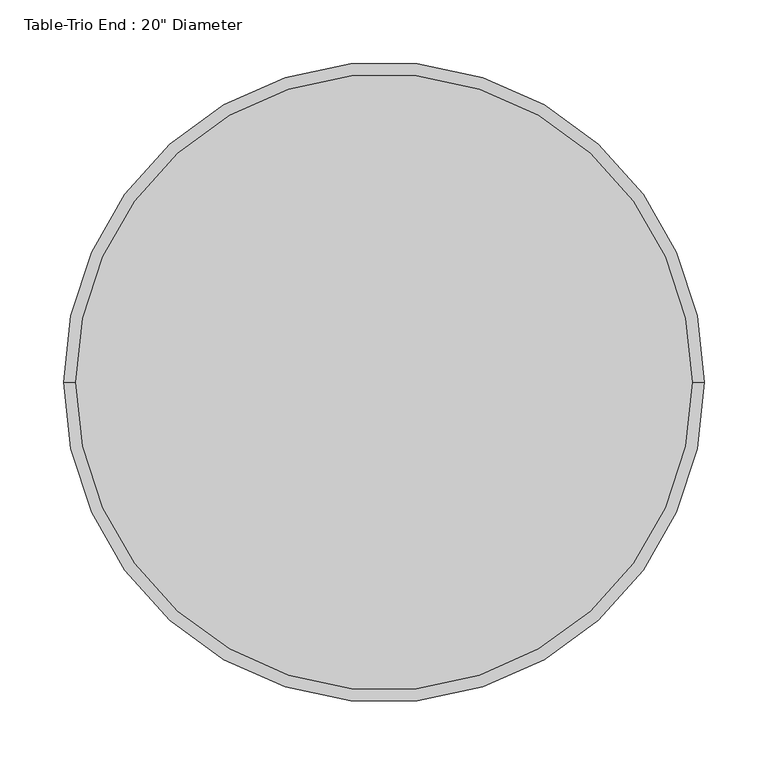
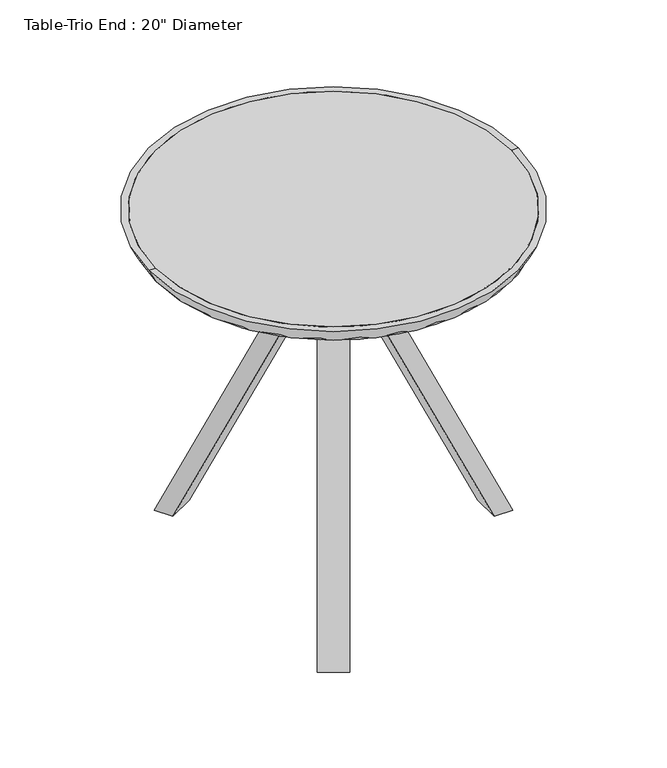
"""IFC4 building model written with IfcOpenShell, lengths in millimetres: furniture geometry."""

from ifc_helpers import new_model, si_unit, point, frame, frame_2d, origin, origin_2d, place, context, project, spatial, polyline, circle_curve, trimmed, segment, composite_curve, outline, extrude, source, transform, mapped, element, save
from ifc_brep_helpers import plane_surface, revolved_surface, advanced_brep


def furniture_3dd5e188(model_context):
    return source(origin(), model_context, "Body", "SolidModel", [
        extrude(outline(composite_curve([segment(trimmed(circle_curve(origin_2d(), 241.3), [point((-241.3, 0.0))], [point((241.3, 0.0))], False, "CARTESIAN"), True, "CONTINUOUS"), segment(trimmed(circle_curve(origin_2d(), 241.3), [point((241.3, 0.0))], [point((-241.3, 0.0))], False, "CARTESIAN"), True, "CONTINUOUS")], self_intersect=False)), frame((0.0, 0.0, 482.6), z_axis=(0.0, 0.0, 1.0), x_axis=(1.0, 0.0, 0.0)), (0.0, 0.0, 1.0), 19.05),
        advanced_brep(
        [(241.3, 0.0, 482.6), (241.3, 0.0, 501.65), (-241.3, 0.0, 501.65), (-241.3, 0.0, 482.6), (250.825, 0.0, 501.65), (-250.825, 0.0, 501.65)],
        [
            (0, 1),
            (1, 2, circle_curve(frame((0.0, 0.0, 501.65), z_axis=(0.0, 0.0, 1.0), x_axis=(-1.0, 0.0, 0.0)), 241.3)),
            (2, 3),
            (3, 0, circle_curve(frame((0.0, 0.0, 482.6), z_axis=(0.0, 0.0, -1.0), x_axis=(-1.0, 0.0, 0.0)), 241.3)),
            (4, 0),
            (3, 5),
            (5, 4, circle_curve(frame((0.0, 0.0, 501.65), z_axis=(0.0, 0.0, -1.0), x_axis=(-1.0, 0.0, 0.0)), 250.825)),
            (1, 4),
            (5, 2),
            (2, 1, circle_curve(frame((0.0, 0.0, 501.65), z_axis=(0.0, 0.0, 1.0), x_axis=(1.0, 0.0, 0.0)), 241.3)),
            (0, 3, circle_curve(frame((0.0, 0.0, 482.6), z_axis=(0.0, 0.0, -1.0), x_axis=(1.0, 0.0, 0.0)), 241.3)),
            (4, 5, circle_curve(frame((0.0, 0.0, 501.65), z_axis=(0.0, 0.0, -1.0), x_axis=(1.0, 0.0, 0.0)), 250.825)),
        ],
        [
            revolved_surface(polyline([(-241.3, 0.0, 501.65), (-241.3, 0.0, 482.6)]), (0.0, 0.0, 0.0), (0.0, 0.0, 1.0)),
            revolved_surface(polyline([(-241.3, 0.0, 482.6), (-250.825, 0.0, 501.65)]), (0.0, 0.0, 0.0), (0.0, 0.0, 1.0)),
            plane_surface(frame((0.0, 0.0, 501.65), z_axis=(0.0, 0.0, 1.0), x_axis=(-1.0, 0.0, 0.0))),
            revolved_surface(polyline([(241.3, 0.0, 501.65), (241.3, 0.0, 482.6)]), (0.0, 0.0, 0.0), (0.0, 0.0, 1.0)),
            revolved_surface(polyline([(241.3, 0.0, 482.6), (250.825, 0.0, 501.65)]), (0.0, 0.0, 0.0), (0.0, 0.0, 1.0)),
            plane_surface(frame((0.0, 0.0, 501.65), z_axis=(0.0, 0.0, 1.0), x_axis=(1.0, 0.0, 0.0))),
        ],
        [
            (0, [[1, 2, 3, 4]]),
            (1, [[5, -4, 6, 7]]),
            (2, [[8, -7, 9, -2]]),
            (3, [[-3, 10, -1, 11]]),
            (4, [[-6, -11, -5, 12]]),
            (5, [[-9, -12, -8, -10]]),
        ],
    ),
        extrude(outline(composite_curve([segment(polyline([(374.1964885, 32.5393466), (0.0, 207.0300348), (0.0, 232.3753669), (384.9309923, 52.8790974)]), True, "CONTINUOUS"), segment(trimmed(circle_curve(frame_2d((406.4, 98.9195329)), 50.8), [point((384.9309923, 52.8790974))], [point((457.2, 98.9195329))], True, "CARTESIAN"), True, "CONTINUOUS"), segment(polyline([(457.2, 98.9195329), (457.2, 154.8312035), (482.6, 154.8312035), (482.6, 101.6)]), True, "CONTINUOUS"), segment(trimmed(circle_curve(frame_2d((406.4, 101.6)), 76.2), [point((482.6, 101.6))], [point((374.1964885, 32.5393466))], False, "CARTESIAN"), True, "CONTINUOUS")], self_intersect=False)), frame((0.0, -19.05, 0.0), z_axis=(0.0, 1.0, 0.0), x_axis=(0.0, 0.0, 1.0)), (0.0, 0.0, 1.0), 38.1),
        extrude(outline(composite_curve([segment(trimmed(circle_curve(frame_2d((-412.8801427, 76.2)), 76.2), [point((-412.8801427, 0.0))], [point((-481.9407961, 108.4035116))], False, "CARTESIAN"), True, "CONTINUOUS"), segment(polyline([(-481.9407961, 108.4035116), (-459.4443174, 156.6473658), (-436.4240996, 145.9128619), (-460.0533926, 95.2396796)]), True, "CONTINUOUS"), segment(trimmed(circle_curve(frame_2d((-414.012957, 73.7706719)), 50.8), [point((-460.0533926, 95.2396796))], [point((-414.0129571, 22.9706718))], True, "CARTESIAN"), True, "CONTINUOUS"), segment(polyline([(-414.0129571, 22.9706718), (10.7114002, 22.9706719), (0.0, 0.0), (-412.8801427, 0.0)]), True, "CONTINUOUS")], self_intersect=False)), frame((-87.0172335, -188.8182695, 0.0), z_axis=(-0.8660254037844397, 0.4999999999999983, 0.0), x_axis=(-0.2113091308703442, -0.36599815077065895, -0.9063077870366545)), (0.0, 0.0, 1.0), 38.1),
        extrude(outline(composite_curve([segment(trimmed(circle_curve(frame_2d((-412.8801427, 76.2)), 76.2), [point((-412.8801427, 0.0))], [point((-481.9407961, 108.4035115))], False, "CARTESIAN"), True, "CONTINUOUS"), segment(polyline([(-481.9407961, 108.4035115), (-459.4443174, 156.6473658), (-436.4240996, 145.9128619), (-460.0533926, 95.2396796)]), True, "CONTINUOUS"), segment(trimmed(circle_curve(frame_2d((-414.012957, 73.7706719)), 50.8), [point((-460.0533926, 95.2396796))], [point((-414.0129571, 22.9706718))], True, "CARTESIAN"), True, "CONTINUOUS"), segment(polyline([(-414.0129571, 22.9706718), (10.7114002, 22.9706719), (0.0, 0.0), (-412.8801427, 0.0)]), True, "CONTINUOUS")], self_intersect=False)), frame((-120.0128014, 169.7682695, 0.0), z_axis=(0.8660254037844366, 0.5000000000000038, 0.0), x_axis=(-0.21130913087034656, 0.3659981507706578, -0.9063077870366544)), (0.0, 0.0, 1.0), 38.1),
        extrude(outline(composite_curve([segment(trimmed(circle_curve(origin_2d(), 31.7871474), [point((-31.7871474, 0.0))], [point((31.7871474, 0.0))], False, "CARTESIAN"), True, "CONTINUOUS"), segment(trimmed(circle_curve(origin_2d(), 31.7871474), [point((31.7871474, 0.0))], [point((-31.7871474, 0.0))], False, "CARTESIAN"), True, "CONTINUOUS")], self_intersect=False)), frame((0.0, 0.0, 381.0), z_axis=(0.0, 0.0, 1.0), x_axis=(1.0, 0.0, 0.0)), (0.0, 0.0, 1.0), 50.8),
    ])


if __name__ == "__main__":
    model = new_model("IFC4")
    model_context = context("Model", 3, world=origin())
    ifc_project = project(units=[si_unit("LENGTHUNIT", "METRE", prefix="MILLI")], contexts=[model_context])
    site = spatial("IfcSite", under=ifc_project)
    building = spatial("IfcBuilding", under=site)
    placement = place(None, origin())
    furniture_shape = furniture_3dd5e188(model_context)
    element("IfcFurniture", 1, ObjectType="Table-Trio End : 20\" Diameter", at=placement, inside=building, context=model_context, shape_type="MappedRepresentation", body=[
        mapped(furniture_shape, transform((0.0, 0.0, 0.0), x_axis=(1.0, 0.0, 0.0), y_axis=(0.0, 1.0, 0.0), z_axis=(0.0, 0.0, 1.0))),
    ])
    save(model, "model.ifc")

# Revit data of these elements
# Type "Table-Trio End : 20\" Diameter"
#   Assembly Code = "E2020200"
#   Base and Trim Material = Wood - Birch
#   Table Top Material = Laminate - Ivory,Matte
#   Default Elevation = 0
# Element 1 (IfcFurniture, "Table-Trio End : 20\" Diameter")
#   Materials on its faces: "Wood - Birch", "Laminate - Ivory,Matte"
# Materials
#   "Wood - Birch": colour RGB 230 196 162, transparency 0
#   "Laminate - Ivory,Matte": colour RGB 127 127 127, transparency 0
